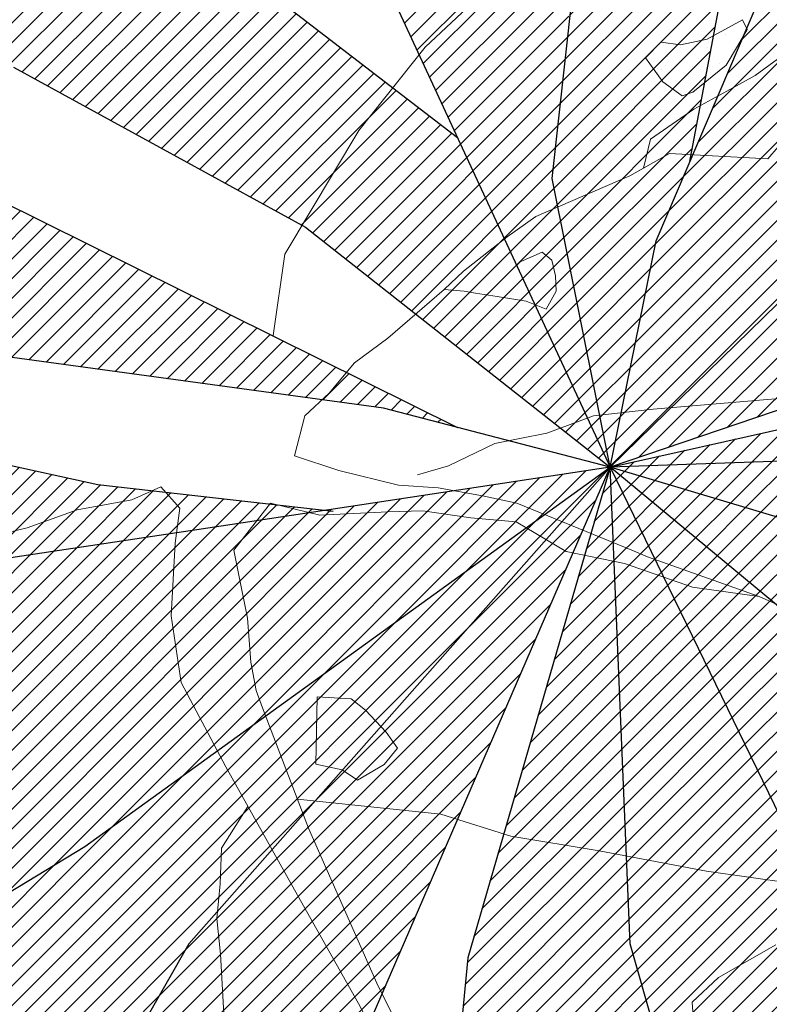
# Model space of a CAD drawing. Units: inches. Extents: x 1986 to 21484, y -1816 to 2016.
# Tile 67 of 85: x 3662.33 to 3670.63, y 1877.89 to 1888.79. Entities that reach past the tile are written whole.
import ezdxf

# ---------------------------------------------------------------- set-up
doc = ezdxf.new("R2010")
doc.units = ezdxf.units.IN
doc.layers.add('L-PLNT', color=84, linetype='Continuous', lineweight=13)
doc.layers.add('vfolhas', color=114, linetype='Continuous', lineweight=5)
for name, color, linetype in [('vfolha', 72, 'Continuous'), ('vfolha2', 110, 'Continuous'), ('vfolhas2', 102, 'Continuous')]:
    doc.layers.add(name, color=color, linetype=linetype)
pattern_1 = [(45, (-2446.5133113, 50.986076), (-0.004419417382, 0.004419417382), [])]

# ---------------------------------------------------------------- blocks, each defined once
blk = doc.blocks.new('arbusto_PB_verde_grande')
at = {"layer": 'vfolha2'}
h = blk.add_hatch(dxfattribs=at)
h.set_pattern_fill('ANSI31', color=256, scale=0.05, style=0)
h.set_pattern_definition(pattern_1)
h.paths.add_polyline_path([(0.02944, 0.35651), (0.00028, 0.09048), (0.02625, -0.03934), (0.047, 0.06233), (0.06189, 0.09731), (0.09372, 0.26573), (0.09955, 0.43473), (0.08789, 0.61313), (0.0645, 0.72266), (0.04988, 0.6851), (0.0236, 0.51294)])
h.paths.add_polyline_path([(0.30106, 0.43789), (0.14225, 0.24871), (0.26685, 0.30022)])
h.paths.add_polyline_path([(0.37995, 0.22817), (0.23697, 0.15193), (0.18428, 0.09364), (0.11122, 0.04358), (0.02625, -0.03934), (0.28061, 0.04667), (0.36829, 0.07798), (0.46756, 0.11239), (0.61068, 0.19376), (0.71585, 0.27823), (0.55813, 0.25948)])
h.paths.add_polyline_path([(0.56101, -0.29441), (0.72752, -0.32573), (0.59024, -0.2412), (0.42962, -0.15982), (0.02625, -0.03934), (0.14922, -0.14107), (0.18838, -0.16604), (0.41501, -0.24435)])
h.paths.add_polyline_path([(-0.27429, -0.44776), (-0.30352, -0.72628), (-0.23923, -0.64175), (-0.15457, -0.45716), (0.02625, -0.03934), (-0.16328, -0.25376)])
h.paths.add_polyline_path([(-0.51963, -0.24744), (-0.67736, -0.32573), (-0.59558, -0.35072), (-0.40574, -0.32882), (-0.21007, -0.20995), (0.02625, -0.03934), (-0.14874, -0.06595), (-0.31518, -0.09101), (-0.41452, -0.15048)])
h.paths.add_polyline_path([(-0.52546, 0.25007), (-0.70947, 0.24698), (-0.51963, 0.1093), (-0.32979, 0.02167), (-0.07567, -0.0128), (-0.04234, -0.02148), (-0.35024, 0.1312)])
h = blk.add_hatch(dxfattribs=at)
h.set_pattern_fill('ANSI31', color=256, scale=0.05, style=0)
h.set_pattern_definition(pattern_1)
h.paths.add_polyline_path([(-0.18963, 0.29704), (-0.08553, 0.20192), (-0.10785, 0.25007), (-0.13202, 0.31865), (-0.25096, 0.48479), (-0.44952, 0.5505), (-0.37946, 0.43789)])
h.paths.add_polyline_path([(0.07911, -0.4071), (0.08214, -0.50631), (0.17255, -0.6355), (0.18428, -0.44151), (0.14904, -0.29177), (0.02625, -0.03934), (0.03527, -0.25376)])
at = {"layer": 'vfolhas'}
h = blk.add_hatch(dxfattribs=at)
h.set_pattern_fill('ANSI31', color=256, scale=0.05, style=0)
h.set_pattern_definition(pattern_1)
h.paths.add_polyline_path([(-0.07279, 0.50669), (-0.18085, 0.65063), (-0.2334, 0.67253), (-0.20712, 0.53176), (-0.10785, 0.25007), (0.02625, -0.03934), (0.00028, 0.09048), (0.00816, 0.16241), (-0.04939, 0.29079)])
h.paths.add_polyline_path([(0.09902, 0.41929), (0.09372, 0.26573), (0.07906, 0.18814), (0.15506, 0.36901), (0.26606, 0.5505), (0.28356, 0.63504), (0.2485, 0.68819), (0.25145, 0.63504), (0.20178, 0.54426)])
h.paths.add_polyline_path([(0.12295, 0.24073), (0.047, 0.06233), (0.02625, -0.03934), (0.11122, 0.04358), (0.18428, 0.09364), (0.27478, 0.19376), (0.3215, 0.25323), (0.44129, 0.38467), (0.47634, 0.57866), (0.41789, 0.45347), (0.28939, 0.30954)])
h.paths.add_polyline_path([(0.58145, -0.03779), (0.70707, 0.01536), (0.78591, 0.04667), (0.74796, 0.06549), (0.62818, 0.08423), (0.52595, 0.09048), (0.39745, 0.04358), (0.02625, -0.03934), (0.25728, -0.03154), (0.43834, -0.0347)])
h.paths.add_polyline_path([(0.52022, -0.03647), (0.43834, -0.0347), (0.25728, -0.03154), (0.02625, -0.03934), (0.17964, -0.08515), (0.53768, -0.13167), (0.69541, -0.15357), (0.78591, -0.07852), (0.70413, -0.10042)])
h.paths.add_polyline_path([(0.27189, -0.21929), (0.14922, -0.14107), (0.02625, -0.03934), (0.15794, -0.31007), (0.29522, -0.42585), (0.41789, -0.49157), (0.56396, -0.56669), (0.5114, -0.48532), (0.39456, -0.34139)])
h.paths.add_polyline_path([(-0.05818, -0.47591), (-0.02312, -0.61984), (0.047, -0.80134), (0.08494, -0.59794), (0.07911, -0.4071), (0.03527, -0.25376), (0.02625, -0.03934), (-0.03773, -0.26001)])
h.paths.add_polyline_path([(-0.24218, 0.14054), (-0.11073, 0.06858), (0.02625, -0.03934), (-0.04235, 0.10871), (-0.21007, 0.23757), (-0.36485, 0.33145), (-0.47874, 0.40341), (-0.54303, 0.46288), (-0.49041, 0.33145), (-0.39408, 0.22192)])
h = blk.add_hatch(dxfattribs=at)
h.set_pattern_fill('ANSI31', color=256, scale=0.05, style=0)
h.set_pattern_definition(pattern_1)
h.paths.add_polyline_path([(-0.57219, 0.06233), (-0.7153, 0.10298), (-0.67736, 0.08107), (-0.62769, 0.01536), (-0.56347, -0.04095), (-0.26461, -0.0834), (-0.14874, -0.06595), (-0.10151, -0.05877), (-0.20418, -0.0472), (-0.40279, -0.00339)])
h.paths.add_polyline_path([(-0.56347, -0.04095), (-0.58279, -0.02401), (-0.72992, -0.09726), (-0.4334, -0.1679), (-0.41452, -0.15048), (-0.31518, -0.09101), (-0.26461, -0.0834)])
h.paths.add_polyline_path([(-0.2769, -0.47267), (-0.27429, -0.44776), (-0.16328, -0.25376), (0.02625, -0.03934), (-0.21007, -0.20995), (-0.2672, -0.24466), (-0.36485, -0.35697), (-0.42907, -0.46341), (-0.47586, -0.60425), (-0.37946, -0.57603)])
at = {"layer": 'vfolha'}
for p, q in [((0.02625, -0.03934), (-0.14874, -0.06595)), ((0.02625, -0.03934), (-0.03773, -0.26001)), ((0.03527, -0.25376), (0.02625, -0.03934)), ((0.07911, -0.4071), (0.03527, -0.25376)), ((-0.03773, -0.26001), (-0.05818, -0.47591))]:
    blk.add_line(p, q, dxfattribs=at)
at = {"layer": 'vfolha2'}
for p, q in [((0.00028, 0.09048), (0.02944, 0.35651)), ((-0.35024, 0.1312), (-0.04234, -0.02148)), ((0.02625, -0.03934), (0.00028, 0.09048)), ((0.28061, 0.04667), (0.02625, -0.03934)), ((-0.07567, -0.0128), (-0.32979, 0.02167)), ((-0.21007, -0.20995), (0.02625, -0.03934)), ((0.02625, -0.03934), (-0.16328, -0.25376)), ((-0.15457, -0.45716), (0.02625, -0.03934)), ((0.42962, -0.15982), (0.02625, -0.03934)), ((0.02625, -0.03934), (0.15794, -0.31007)), ((-0.14874, -0.06595), (-0.31518, -0.09101)), ((-0.40574, -0.32882), (-0.21007, -0.20995)), ((-0.16328, -0.25376), (-0.27429, -0.44776))]:
    blk.add_line(p, q, dxfattribs=at)
at = {"layer": 'vfolhas2'}
for p, q in [((0.09372, 0.26573), (0.06189, 0.09731)), ((-0.10785, 0.25007), (0.02625, -0.03934)), ((0.047, 0.06233), (0.12295, 0.24073)), ((-0.04235, 0.10871), (-0.21007, 0.23757)), ((-0.24218, 0.14054), (-0.11073, 0.06858)), ((-0.11073, 0.06858), (0.02625, -0.03934)), ((0.02625, -0.03934), (0.047, 0.06233)), ((0.02625, -0.03934), (0.39745, 0.04358)), ((0.11122, 0.04358), (0.02625, -0.03934)), ((-0.40279, -0.00339), (-0.20418, -0.0472)), ((0.02625, -0.03934), (-0.07567, -0.0128)), ((0.25728, -0.03154), (0.02625, -0.03934)), ((0.14922, -0.14107), (0.02625, -0.03934)), ((-0.20418, -0.0472), (-0.09832, -0.05913))]:
    blk.add_line(p, q, dxfattribs=at)
blk = doc.blocks.new('PLANT-SHRUB')
for p, q in [((2166.425, 1895.077), (2167.137, 1894.905)), ((2167.534, 1894.905), (2167.727, 1895.138)), ((2167.137, 1894.905), (2167.534, 1894.905)), ((2166.428, 1893.958), (2165.771, 1894.775)), ((2169.936, 1892.362), (2170.509, 1894.276)), ((2167.138, 1892.979), (2166.428, 1893.958)), ((2170.489, 1893.314), (2170.238, 1892.387)), ((2163.924, 1892.139), (2163.483, 1893.181)), ((2167.741, 1892.194), (2167.138, 1892.979)), ((2169.314, 1890.595), (2169.936, 1892.362)), ((2170.238, 1892.387), (2169.893, 1890.986)), ((2163.924, 1892.139), (2164.39, 1891.561)), ((2164.525, 1890.975), (2163.924, 1892.139)), ((2168.139, 1891.484), (2167.741, 1892.194)), ((2164.39, 1891.561), (2164.759, 1890.854)), ((2169.185, 1890.278), (2168.139, 1891.484)), ((2170.979, 1890.943), (2171.402, 1891.45)), ((2161.819, 1891.046), (2163.359, 1889.824)), ((2164.599, 1890.803), (2164.525, 1890.975)), ((2169.893, 1890.986), (2169.518, 1889.474)), ((2170.737, 1890.629), (2170.979, 1890.943)), ((2164.759, 1890.854), (2165.138, 1890.314)), ((2165.17, 1889.552), (2164.599, 1890.803)), ((2167.96, 1890.411), (2167.99, 1890.624)), ((2167.99, 1890.624), (2168.22, 1890.655)), ((2168.22, 1890.655), (2168.556, 1890.579)), ((2170.447, 1890.376), (2170.737, 1890.629)), ((2168.181, 1890.506), (2168.181, 1890.506)), ((2168.461, 1890.556), (2168.461, 1890.556)), ((2168.556, 1890.579), (2168.602, 1890.38)), ((2168.774, 1889.274), (2169.314, 1890.595)), ((2167.96, 1890.074), (2167.96, 1890.411)), ((2168.287, 1890.397), (2168.287, 1890.397)), ((2165.138, 1890.314), (2165.318, 1889.697)), ((2168.149, 1890.329), (2168.149, 1890.329)), ((2168.251, 1890.363), (2168.251, 1890.363)), ((2168.422, 1890.321), (2168.422, 1890.321)), ((2168.602, 1890.38), (2168.77, 1890.135)), ((2168.602, 1890.38), (2168.602, 1890.38)), ((2170.169, 1890.098), (2170.447, 1890.376)), ((2168.052, 1890.181), (2168.052, 1890.181)), ((2168.063, 1890.25), (2168.063, 1890.25)), ((2168.167, 1890.236), (2168.167, 1890.236)), ((2168.33, 1890.215), (2168.33, 1890.215)), ((2168.601, 1890.179), (2168.601, 1890.179)), ((2167.99, 1889.876), (2167.96, 1890.074)), ((2168.169, 1890.121), (2168.169, 1890.121)), ((2168.77, 1890.135), (2168.25, 1889.601)), ((2168.384, 1890.081), (2168.384, 1890.081)), ((2168.468, 1890.135), (2168.468, 1890.135)), ((2168.692, 1890.114), (2168.692, 1890.114)), ((2168.705, 1890.165), (2168.705, 1890.165)), ((2169.639, 1889.962), (2170.169, 1890.098)), ((2169.639, 1889.962), (2169.639, 1889.962)), ((2168.25, 1889.601), (2167.99, 1889.876)), ((2168.41, 1889.936), (2168.41, 1889.936)), ((2168.479, 1889.846), (2168.479, 1889.846)), ((2163.359, 1889.824), (2163.892, 1889.429)), ((2168.442, 1889.813), (2168.442, 1889.813)), ((2165.318, 1889.697), (2165.652, 1889.321)), ((2168.145, 1889.721), (2168.145, 1889.721)), ((2168.156, 1889.736), (2168.156, 1889.736)), ((2168.243, 1889.63), (2168.243, 1889.63)), ((2165.393, 1889.23), (2165.17, 1889.552)), ((2163.892, 1889.429), (2164.399, 1889.214)), ((2169.518, 1889.474), (2169.239, 1888.457)), ((2165.652, 1889.321), (2165.986, 1888.901)), ((2164.399, 1889.214), (2164.657, 1889.051)), ((2165.393, 1889.23), (2165.393, 1889.23)), ((2165.691, 1888.833), (2165.393, 1889.23)), ((2168.694, 1889.087), (2168.774, 1889.274)), ((2168.521, 1888.82), (2168.694, 1889.087)), ((2164.657, 1889.051), (2164.897, 1888.905)), ((2164.897, 1888.905), (2165.439, 1888.733)), ((2165.986, 1888.901), (2166.278, 1888.644)), ((2165.989, 1888.51), (2165.691, 1888.833)), ((2168.214, 1888.439), (2168.521, 1888.82)), ((2160.54, 1888.674), (2160.191, 1888.639)), ((2161.292, 1887.888), (2160.54, 1888.674)), ((2165.439, 1888.733), (2165.757, 1888.57)), ((2166.278, 1888.644), (2166.852, 1888.156)), ((2166.362, 1887.939), (2165.989, 1888.51)), ((2167.94, 1887.993), (2168.214, 1888.439)), ((2169.239, 1888.457), (2168.816, 1887.842)), ((2163.248, 1888.139), (2163.136, 1888.01)), ((2163.464, 1888.209), (2163.248, 1888.139)), ((2163.567, 1887.993), (2163.464, 1888.209)), ((2166.852, 1888.156), (2167.16, 1887.685)), ((2163.136, 1888.01), (2163.049, 1887.855)), ((2160.01, 1887.906), (2159.433, 1887.976)), ((2160.359, 1887.819), (2160.01, 1887.906)), ((2161.781, 1887.766), (2161.292, 1887.888)), ((2163.766, 1887.734), (2163.567, 1887.993)), ((2166.362, 1887.939), (2166.362, 1887.939)), ((2166.606, 1887.486), (2166.362, 1887.939)), ((2167.812, 1887.788), (2167.94, 1887.993)), ((2160.761, 1887.714), (2160.359, 1887.819)), ((2161.611, 1887.808), (2161.338, 1887.627)), ((2161.781, 1887.766), (2161.611, 1887.808)), ((2163.049, 1887.855), (2163.067, 1887.717)), ((2167.16, 1887.685), (2167.812, 1887.788)), ((2168.816, 1887.842), (2168.231, 1887.286)), ((2161.338, 1887.627), (2160.761, 1887.714)), ((2162.848, 1887.381), (2161.781, 1887.766)), ((2163.067, 1887.717), (2163.317, 1887.63)), ((2163.913, 1887.544), (2163.766, 1887.734)), ((2160.165, 1887.605), (2159.932, 1887.536)), ((2160.64, 1887.57), (2160.165, 1887.605)), ((2160.753, 1887.518), (2160.64, 1887.57)), ((2163.317, 1887.63), (2163.421, 1887.63)), ((2159.725, 1887.475), (2159.69, 1887.363)), ((2159.932, 1887.536), (2159.725, 1887.475)), ((2160.21, 1887.544), (2160.21, 1887.544)), ((2160.351, 1887.48), (2160.351, 1887.48)), ((2160.804, 1887.259), (2160.753, 1887.518)), ((2163.991, 1887.441), (2163.913, 1887.544)), ((2166.606, 1887.486), (2166.221, 1887.242)), ((2159.69, 1887.363), (2160.122, 1887.251)), ((2159.94, 1887.356), (2159.94, 1887.356)), ((2160.451, 1887.359), (2160.451, 1887.359)), ((2163.232, 1887.329), (2162.848, 1887.381)), ((2164.141, 1887.277), (2163.991, 1887.441)), ((2160.122, 1887.251), (2160.381, 1887.095)), ((2160.141, 1887.287), (2160.141, 1887.287)), ((2160.177, 1887.321), (2160.177, 1887.321)), ((2160.335, 1887.339), (2160.335, 1887.339)), ((2160.761, 1886.932), (2160.804, 1887.259)), ((2163.844, 1887.277), (2163.232, 1887.329)), ((2164.141, 1887.277), (2163.844, 1887.277)), ((2164.963, 1887.242), (2164.141, 1887.277)), ((2165.417, 1887.189), (2164.963, 1887.242)), ((2165.854, 1887.242), (2165.417, 1887.189)), ((2165.854, 1887.242), (2165.854, 1887.242)), ((2166.221, 1887.242), (2165.854, 1887.242)), ((2168.231, 1887.286), (2167.929, 1887.04)), ((2160.654, 1887.145), (2160.654, 1887.145)), ((2160.721, 1887.152), (2160.721, 1887.152)), ((2160.778, 1887.146), (2160.778, 1887.146)), ((2160.381, 1887.095), (2160.519, 1886.923)), ((2160.401, 1887.119), (2160.401, 1887.119)), ((2160.57, 1887.091), (2160.57, 1887.091)), ((2160.672, 1887.084), (2160.672, 1887.084)), ((2160.741, 1887.112), (2160.741, 1887.112)), ((2160.776, 1887.07), (2160.776, 1887.07)), ((2167.929, 1887.04), (2167.921, 1886.722)), ((2160.519, 1886.923), (2160.761, 1886.932)), ((2160.542, 1886.93), (2160.542, 1886.93)), ((2167.921, 1886.722), (2168.255, 1886.608)), ((2168.255, 1886.608), (2168.771, 1886.274)), ((2165.16, 1885.786), (2165.869, 1886.351)), ((2168.771, 1886.274), (2169.31, 1886.039)), ((2169.31, 1886.039), (2169.765, 1885.781)), ((2163.626, 1885.349), (2165.16, 1885.786)), ((2162.459, 1885.179), (2163.626, 1885.349)), ((2161.17, 1885.179), (2162.459, 1885.179))]:
    blk.add_line(p, q)

msp = doc.modelspace()

# ---------------------------------------------------------------- block references
at = {"layer": 'L-PLNT', "rotation": 223.1883365522388}
msp.add_blockref('PLANT-SHRUB', (3953.27, 4742.965), dxfattribs=at)
at = {"layer": 'L-PLNT', "xscale": 24.60366729364114, "yscale": 24.60366729364114, "zscale": 24.60366729364114}
msp.add_blockref('arbusto_PB_verde_grande', (3668.218, 1884.805), dxfattribs=at)

doc.saveas('drawing.dxf')
